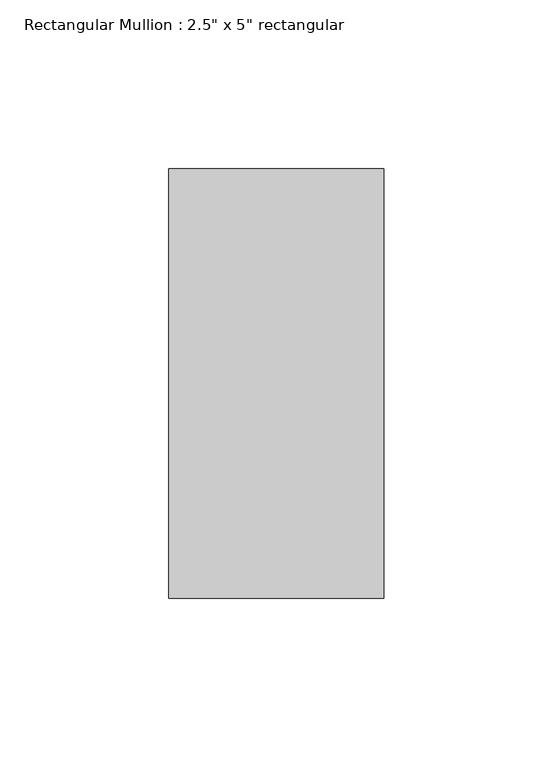
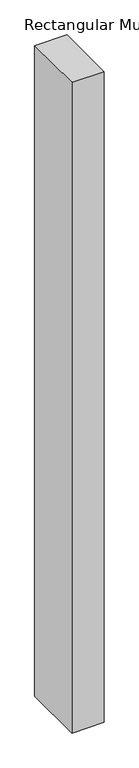
"""IFC4 building model written with IfcOpenShell, lengths in millimetres: member geometry."""

from ifc_helpers import new_model, si_unit, frame, origin, place, context, project, spatial, polyline, outline, extrude, source, transform, mapped, element, save


def member_21317375(model_context):
    return source(origin(), model_context, "Body", "SweptSolid", [
        extrude(outline(polyline([(31.75, 63.5), (31.75, -63.5), (-31.75, -63.5), (-31.75, 63.5), (31.75, 63.5)])), frame((0.0, 0.0, -1359.7734608), z_axis=(0.0, 0.0, 1.0), x_axis=(1.0, 0.0, 0.0)), (0.0, 0.0, 1.0), 1359.7734608),
    ])


if __name__ == "__main__":
    model = new_model("IFC4")
    model_context = context("Model", 3, world=origin())
    ifc_project = project(units=[si_unit("LENGTHUNIT", "METRE", prefix="MILLI")], contexts=[model_context])
    site = spatial("IfcSite", under=ifc_project)
    building = spatial("IfcBuilding", under=site)
    placement = place(None, origin())
    member_shape = member_21317375(model_context)
    element("IfcMember", 1, ObjectType="Rectangular Mullion : 2.5\" x 5\" rectangular", at=placement, inside=building, context=model_context, shape_type="MappedRepresentation", body=[
        mapped(member_shape, transform((0.0, 0.0, 0.0), x_axis=(1.0, 0.0, 0.0), y_axis=(0.0, 1.0, 0.0), z_axis=(0.0, 0.0, 1.0))),
    ])
    save(model, "model.ifc")

# Revit data of these elements
# Type "Rectangular Mullion : 2.5\" x 5\" rectangular"
#   built-in parameter 1007304 = 0.416667 (stored number, unit not read)
#   built-in parameter 1007301 = 0.104167 (stored number, unit not read)
#   built-in parameter 1007300 = 0.104167 (stored number, unit not read)
# Element 1 (IfcMember, "Rectangular Mullion : 2.5\" x 5\" rectangular")
#   Materials on its faces: "Aluminum"
# Materials
#   "Aluminum": class "Metal", colour RGB 247 247 247, transparency 0, Description = "Aluminum 6061", Cost = 0
